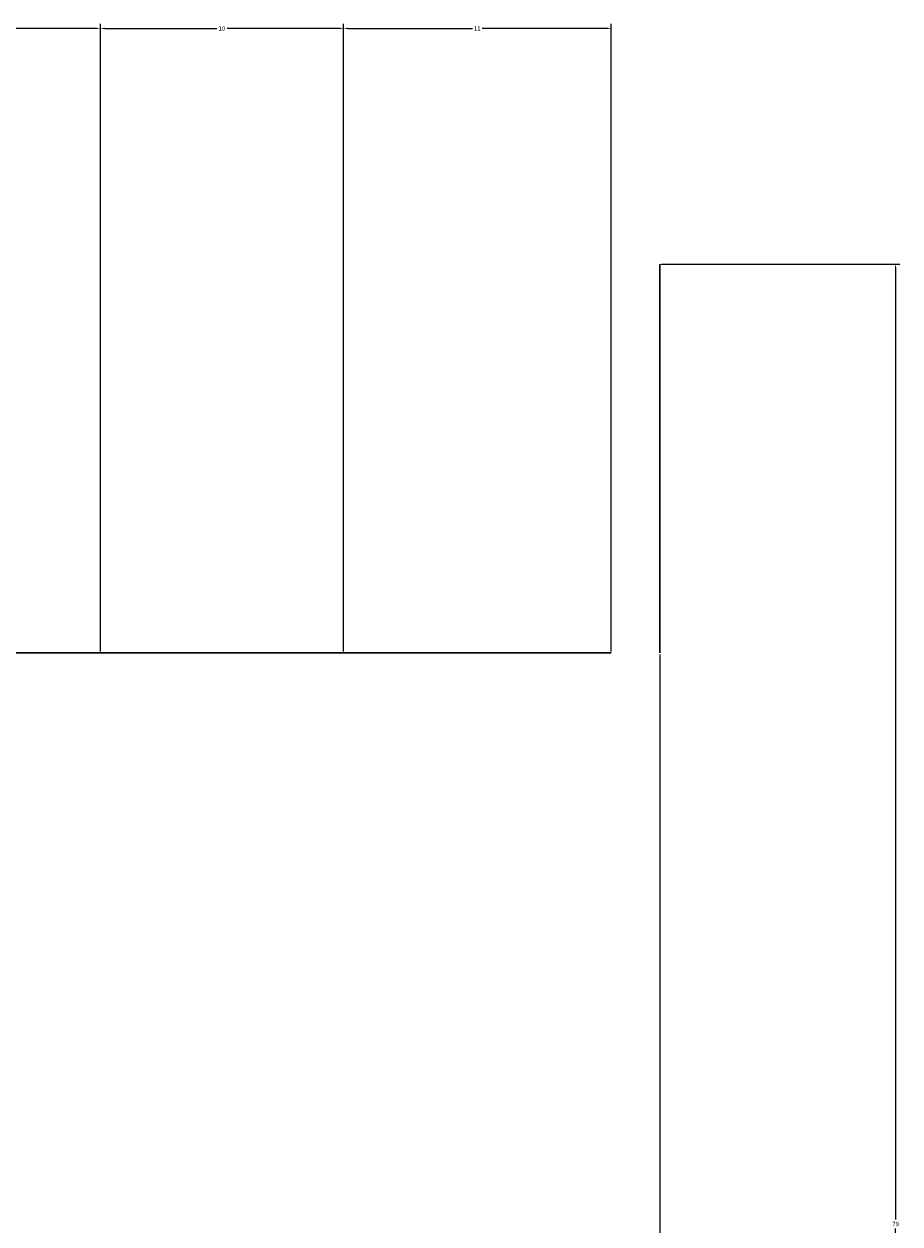
# Model space of a CAD drawing. Units: millimetres. Extents: x -136 to 10, y 158 to 257.
# Tile 6 of 6: x -26 to 10, y 208 to 257. Entities that reach past the tile are written whole.
import ezdxf

# ---------------------------------------------------------------- set-up
doc = ezdxf.new("R2010")
doc.units = ezdxf.units.MM
doc.layers.add('M-CONS', color=8, linetype='Continuous', lineweight=18)
doc.layers.add('M-DIMS', color=2, linetype='Continuous', lineweight=18)
doc.styles.get("Standard").update_dxf_attribs({"font": 'arial.ttf'})
doc.dimstyles.get("Standard").update_dxf_attribs({"dimtxt": 0.18, "dimasz": 0.18, "dimexe": 0.18, "dimexo": 0.0625, "dimgap": 0.09, "dimtad": 0, "dimtih": 1, "dimtoh": 1, "dimdec": 4, "dimzin": 0, "dimdsep": 46, "dimtxsty": 'Standard', "dimcen": 0.09, "dimadec": 0, "dimazin": 0, "dimtfac": 1, "dimtdec": 4, "dimtofl": 0, "dimtmove": 0, "dimatfit": 3, "dimfxl": 1, "dimtolj": 1, "dimtzin": 0, "dimarcsym": 0})

# ---------------------------------------------------------------- blocks, each defined once
blk = doc.blocks.new('*D1')
at = {"layer": 'Defpoints', "color": 0, "transparency": 16777216}
for p in [(-126, 231.107), (0, 231.107), (0, 158.407)]:
    blk.add_point(p, dxfattribs=at)
at = {"layer": 'M-DIMS', "color": 0, "lineweight": -2, "transparency": 16777216}
for p, q in [((-126, 231.044), (-126, 158.227)), ((0, 231.044), (0, 158.227)), ((-125.82, 158.407), (-63.28, 158.407)), ((-0.18, 158.407), (-62.72, 158.407))]:
    blk.add_line(p, q, dxfattribs=at)
at = {"layer": 'M-DIMS', "color": 0, "transparency": 16777216}
for points in [[(-125.82, 158.437), (-125.82, 158.377), (-126, 158.407)], [(-0.18, 158.437), (-0.18, 158.377), (0, 158.407)]]:
    blk.add_solid(points, dxfattribs=at)
at = {"layer": 'M-DIMS', "color": 0, "transparency": 16777216, "insert": (-63, 158.407), "char_height": 0.18, "attachment_point": 5}
blk.add_mtext('\\A1;126', dxfattribs=at)
blk = doc.blocks.new('*D2')
at = {"layer": 'Defpoints', "color": 0, "transparency": 16777216}
for p in [(0, 247.107), (9.7, 247.107), (-62.158, 168.107)]:
    blk.add_point(p, dxfattribs=at)
at = {"layer": 'M-DIMS', "color": 0, "lineweight": -2, "transparency": 16777216}
for p, q in [((0.062, 247.107), (9.88, 247.107)), ((9.7, 246.927), (9.7, 207.789)), ((9.7, 168.287), (9.7, 207.425)), ((-62.095, 168.107), (9.88, 168.107))]:
    blk.add_line(p, q, dxfattribs=at)
at = {"layer": 'M-DIMS', "color": 0, "transparency": 16777216}
for points in [[(9.67, 246.927), (9.73, 246.927), (9.7, 247.107)], [(9.67, 168.287), (9.73, 168.287), (9.7, 168.107)]]:
    blk.add_solid(points, dxfattribs=at)
at = {"layer": 'M-DIMS', "color": 0, "transparency": 16777216, "insert": (9.7, 207.607), "char_height": 0.18, "attachment_point": 5}
blk.add_mtext('\\A1;79', dxfattribs=at)
blk = doc.blocks.new('*D11')
at = {"layer": 'Defpoints', "color": 0, "transparency": 16777216}
for p in [(-23, 256.807), (-34, 231.107), (-23, 231.107)]:
    blk.add_point(p, dxfattribs=at)
at = {"layer": 'M-DIMS', "color": 0, "lineweight": -2, "transparency": 16777216}
for p, q in [((-34, 231.169), (-34, 256.987)), ((-33.82, 256.807), (-28.693, 256.807)), ((-23.18, 256.807), (-28.307, 256.807)), ((-23, 231.169), (-23, 256.987))]:
    blk.add_line(p, q, dxfattribs=at)
at = {"layer": 'M-DIMS', "color": 0, "transparency": 16777216}
for points in [[(-33.82, 256.837), (-33.82, 256.777), (-34, 256.807)], [(-23.18, 256.837), (-23.18, 256.777), (-23, 256.807)]]:
    blk.add_solid(points, dxfattribs=at)
at = {"layer": 'M-DIMS', "color": 0, "transparency": 16777216, "insert": (-28.5, 256.807), "char_height": 0.18, "attachment_point": 5}
blk.add_mtext('\\A1;11', dxfattribs=at)
blk = doc.blocks.new('*D12')
at = {"layer": 'Defpoints', "color": 0, "transparency": 16777216}
for p in [(-13, 256.807), (-23, 231.107), (-13, 231.107)]:
    blk.add_point(p, dxfattribs=at)
at = {"layer": 'M-DIMS', "color": 0, "lineweight": -2, "transparency": 16777216}
for p, q in [((-23, 231.169), (-23, 256.987)), ((-22.82, 256.807), (-18.21, 256.807)), ((-13.18, 256.807), (-17.79, 256.807)), ((-13, 231.169), (-13, 256.987))]:
    blk.add_line(p, q, dxfattribs=at)
at = {"layer": 'M-DIMS', "color": 0, "transparency": 16777216}
for points in [[(-22.82, 256.837), (-22.82, 256.777), (-23, 256.807)], [(-13.18, 256.837), (-13.18, 256.777), (-13, 256.807)]]:
    blk.add_solid(points, dxfattribs=at)
at = {"layer": 'M-DIMS', "color": 0, "transparency": 16777216, "insert": (-18, 256.807), "char_height": 0.18, "attachment_point": 5}
blk.add_mtext('\\A1;10', dxfattribs=at)
blk = doc.blocks.new('*D13')
at = {"layer": 'Defpoints', "color": 0, "transparency": 16777216}
for p in [(-2, 256.807), (-13, 231.107), (-2, 231.107)]:
    blk.add_point(p, dxfattribs=at)
at = {"layer": 'M-DIMS', "color": 0, "lineweight": -2, "transparency": 16777216}
for p, q in [((-13, 231.169), (-13, 256.987)), ((-12.82, 256.807), (-7.693, 256.807)), ((-2.18, 256.807), (-7.307, 256.807)), ((-2, 231.169), (-2, 256.987))]:
    blk.add_line(p, q, dxfattribs=at)
at = {"layer": 'M-DIMS', "color": 0, "transparency": 16777216}
for points in [[(-12.82, 256.837), (-12.82, 256.777), (-13, 256.807)], [(-2.18, 256.837), (-2.18, 256.777), (-2, 256.807)]]:
    blk.add_solid(points, dxfattribs=at)
at = {"layer": 'M-DIMS', "color": 0, "transparency": 16777216, "insert": (-7.5, 256.807), "char_height": 0.18, "attachment_point": 5}
blk.add_mtext('\\A1;11', dxfattribs=at)

msp = doc.modelspace()

# ---------------------------------------------------------------- linework, layer by layer
at = {"layer": 'M-CONS', "extrusion": (1, 0, 0)}
msp.add_lwpolyline([(231.1068, 68.8035), (231.1068, 128.8035), (247.1068, 128.8035), (247.1068, 118.8035), (244.1068, 118.8035), (244.1068, 78.8035), (247.1068, 78.8035), (247.1068, 68.8035)], close=True, dxfattribs=at)
at = {"layer": 'M-CONS', "extrusion": (0, -1, 0)}
for radius in [16, 5]:
    msp.add_circle((-18, 98.8035, -231.1068), radius, dxfattribs=at)

# ---------------------------------------------------------------- dimensions: what is measured, and where the dimension line sits
at = {"layer": 'M-DIMS'}
for base, p1, p2, picture, middle in [((-23, 256.8068), (-34, 231.1068), (-23, 231.1068), '*D11', (-28.5, 256.8068)), ((-13, 256.8068), (-23, 231.1068), (-13, 231.1068), '*D12', (-18, 256.8068)), ((-2, 256.8068), (-13, 231.1068), (-2, 231.1068), '*D13', (-7.5, 256.8068)), ((0, 158.4068), (-126, 231.1068), (0, 231.1068), '*D1', (-63, 158.4068))]:
    dim = msp.add_linear_dim(base=base, p1=p1, p2=p2, dimstyle='Standard', override={"dimdec": 0, "dimlfac": 1, "dimrnd": 0, "dimzin": 0, "dimdsep": 46, "dimlunit": 2}, dxfattribs=at)
    dim.commit()
    dim.dimension.update_dxf_attribs({"geometry": picture, "text_midpoint": middle})
dim = msp.add_linear_dim(base=(9.7, 247.1068), p1=(-62.158, 168.1068), p2=(0, 247.1068), angle=90, dimstyle='Standard', override={"dimdec": 0, "dimlfac": 1, "dimrnd": 0, "dimzin": 0, "dimdsep": 46, "dimlunit": 2}, dxfattribs=at)
dim.commit()
dim.dimension.update_dxf_attribs({"geometry": '*D2', "text_midpoint": (9.7, 207.6068)})

doc.saveas('drawing.dxf')
